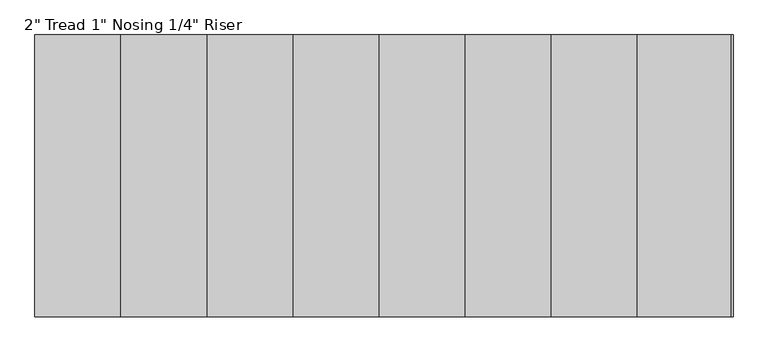
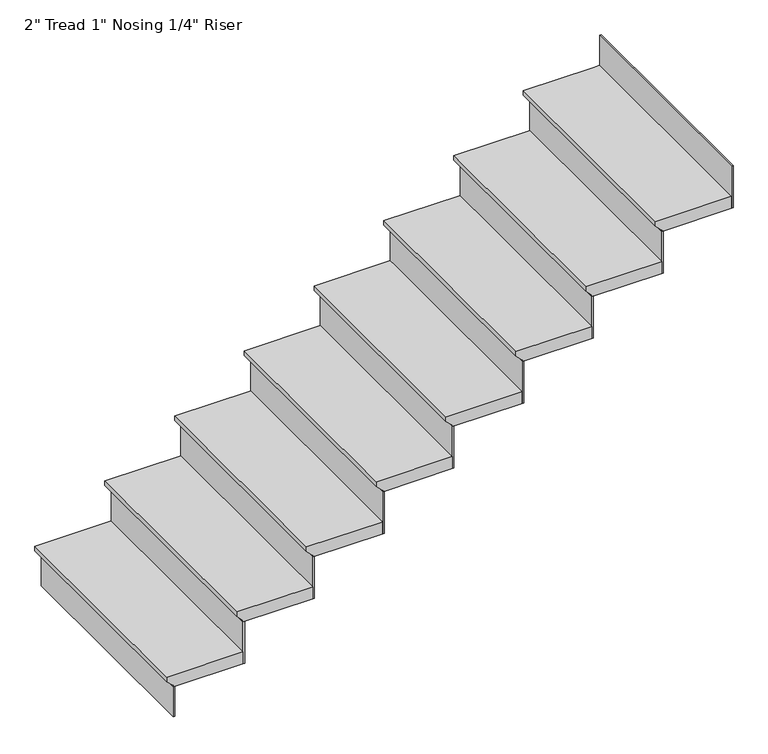
"""IFC4 building model written with IfcOpenShell, lengths in millimetres: stair flight geometry."""

from ifc_helpers import new_model, si_unit, origin, place, context, project, spatial, faceted_brep, source, transform, mapped, element, save


def stair_flight_350f2e97(model_context):
    return source(origin(), model_context, "Body", "Brep", [
        faceted_brep([(-4413.813859, 444.1428136, 158.75), (-4413.813859, 444.1428136, 177.8), (-4413.813859, 1358.5428136, 177.8), (-4413.813859, 1358.5428136, 158.75), (-4388.413859, 444.1428136, 133.35), (-4388.413859, 1358.5428136, 133.35), (-4109.013859, 444.1428136, 177.8), (-4109.013859, 1358.5428136, 177.8), (-4388.413859, 1358.5428136, 127.0), (-4109.013859, 1358.5428136, 127.0), (-4109.013859, 444.1428136, 127.0), (-4388.413859, 444.1428136, 127.0)], [[[0, 1, 2, 3]], [[4, 0, 3, 5]], [[2, 1, 6, 7]], [[8, 9, 10, 11]], [[2, 7, 9, 8, 5, 3]], [[8, 11, 4, 5]], [[6, 1, 0, 4, 11, 10]], [[7, 6, 10, 9]]]),
        faceted_brep([(-4388.413859, 444.1428136, 127.0), (-4388.413859, 444.1428136, 0.0), (-4382.063859, 444.1428136, 0.0), (-4382.063859, 444.1428136, 127.0), (-4388.413859, 1358.5428136, 127.0), (-4382.063859, 1358.5428136, 127.0), (-4382.063859, 1358.5428136, 0.0), (-4388.413859, 1358.5428136, 0.0)], [[[0, 1, 2, 3]], [[4, 5, 6, 7]], [[1, 0, 4, 7]], [[2, 1, 7, 6]], [[3, 2, 6, 5]], [[0, 3, 5, 4]]]),
        faceted_brep([(-4109.013859, 444.1428136, 304.8), (-4109.013859, 444.1428136, 127.0), (-4102.663859, 444.1428136, 127.0), (-4102.663859, 444.1428136, 304.8), (-4109.013859, 1358.5428136, 304.8), (-4102.663859, 1358.5428136, 304.8), (-4102.663859, 1358.5428136, 127.0), (-4109.013859, 1358.5428136, 127.0)], [[[0, 1, 2, 3]], [[4, 5, 6, 7]], [[1, 0, 4, 7]], [[2, 1, 7, 6]], [[3, 2, 6, 5]], [[0, 3, 5, 4]]]),
        faceted_brep([(-4134.413859, 1358.5428136, 355.6), (-4134.413859, 444.1428136, 355.6), (-3829.613859, 444.1428136, 355.6), (-3829.613859, 1358.5428136, 355.6), (-4109.013859, 1358.5428136, 304.8), (-3829.613859, 1358.5428136, 304.8), (-3829.613859, 444.1428136, 304.8), (-4109.013859, 444.1428136, 304.8), (-4109.013859, 1358.5428136, 311.15), (-4134.413859, 1358.5428136, 336.55), (-4109.013859, 444.1428136, 311.15), (-4134.413859, 444.1428136, 336.55)], [[[0, 1, 2, 3]], [[4, 5, 6, 7]], [[0, 3, 5, 4, 8, 9]], [[4, 7, 10, 8]], [[2, 1, 11, 10, 7, 6]], [[3, 2, 6, 5]], [[11, 1, 0, 9]], [[10, 11, 9, 8]]]),
        faceted_brep([(-3829.613859, 444.1428136, 482.6), (-3829.613859, 444.1428136, 304.8), (-3823.263859, 444.1428136, 304.8), (-3823.263859, 444.1428136, 482.6), (-3829.613859, 1358.5428136, 482.6), (-3823.263859, 1358.5428136, 482.6), (-3823.263859, 1358.5428136, 304.8), (-3829.613859, 1358.5428136, 304.8)], [[[0, 1, 2, 3]], [[4, 5, 6, 7]], [[1, 0, 4, 7]], [[2, 1, 7, 6]], [[3, 2, 6, 5]], [[0, 3, 5, 4]]]),
        faceted_brep([(-3855.013859, 1358.5428136, 533.4), (-3855.013859, 444.1428136, 533.4), (-3550.213859, 444.1428136, 533.4), (-3550.213859, 1358.5428136, 533.4), (-3829.613859, 1358.5428136, 482.6), (-3550.213859, 1358.5428136, 482.6), (-3550.213859, 444.1428136, 482.6), (-3829.613859, 444.1428136, 482.6), (-3829.613859, 1358.5428136, 488.95), (-3855.013859, 1358.5428136, 514.35), (-3829.613859, 444.1428136, 488.95), (-3855.013859, 444.1428136, 514.35)], [[[0, 1, 2, 3]], [[4, 5, 6, 7]], [[0, 3, 5, 4, 8, 9]], [[4, 7, 10, 8]], [[2, 1, 11, 10, 7, 6]], [[3, 2, 6, 5]], [[11, 1, 0, 9]], [[10, 11, 9, 8]]]),
        faceted_brep([(-3550.213859, 444.1428136, 660.4), (-3550.213859, 444.1428136, 482.6), (-3543.863859, 444.1428136, 482.6), (-3543.863859, 444.1428136, 660.4), (-3550.213859, 1358.5428136, 660.4), (-3543.863859, 1358.5428136, 660.4), (-3543.863859, 1358.5428136, 482.6), (-3550.213859, 1358.5428136, 482.6)], [[[0, 1, 2, 3]], [[4, 5, 6, 7]], [[1, 0, 4, 7]], [[2, 1, 7, 6]], [[3, 2, 6, 5]], [[0, 3, 5, 4]]]),
        faceted_brep([(-3575.613859, 1358.5428136, 711.2), (-3575.613859, 444.1428136, 711.2), (-3270.813859, 444.1428136, 711.2), (-3270.813859, 1358.5428136, 711.2), (-3550.213859, 1358.5428136, 660.4), (-3270.813859, 1358.5428136, 660.4), (-3270.813859, 444.1428136, 660.4), (-3550.213859, 444.1428136, 660.4), (-3550.213859, 1358.5428136, 666.75), (-3575.613859, 1358.5428136, 692.15), (-3550.213859, 444.1428136, 666.75), (-3575.613859, 444.1428136, 692.15)], [[[0, 1, 2, 3]], [[4, 5, 6, 7]], [[0, 3, 5, 4, 8, 9]], [[4, 7, 10, 8]], [[2, 1, 11, 10, 7, 6]], [[3, 2, 6, 5]], [[11, 1, 0, 9]], [[10, 11, 9, 8]]]),
        faceted_brep([(-3270.813859, 444.1428136, 838.2), (-3270.813859, 444.1428136, 660.4), (-3264.463859, 444.1428136, 660.4), (-3264.463859, 444.1428136, 838.2), (-3270.813859, 1358.5428136, 838.2), (-3264.463859, 1358.5428136, 838.2), (-3264.463859, 1358.5428136, 660.4), (-3270.813859, 1358.5428136, 660.4)], [[[0, 1, 2, 3]], [[4, 5, 6, 7]], [[1, 0, 4, 7]], [[2, 1, 7, 6]], [[3, 2, 6, 5]], [[0, 3, 5, 4]]]),
        faceted_brep([(-3296.213859, 1358.5428136, 889.0), (-3296.213859, 444.1428136, 889.0), (-2991.413859, 444.1428136, 889.0), (-2991.413859, 1358.5428136, 889.0), (-3270.813859, 1358.5428136, 838.2), (-2991.413859, 1358.5428136, 838.2), (-2991.413859, 444.1428136, 838.2), (-3270.813859, 444.1428136, 838.2), (-3270.813859, 1358.5428136, 844.55), (-3296.213859, 1358.5428136, 869.95), (-3270.813859, 444.1428136, 844.55), (-3296.213859, 444.1428136, 869.95)], [[[0, 1, 2, 3]], [[4, 5, 6, 7]], [[0, 3, 5, 4, 8, 9]], [[4, 7, 10, 8]], [[2, 1, 11, 10, 7, 6]], [[3, 2, 6, 5]], [[11, 1, 0, 9]], [[10, 11, 9, 8]]]),
        faceted_brep([(-2991.413859, 444.1428136, 1016.0), (-2991.413859, 444.1428136, 838.2), (-2985.063859, 444.1428136, 838.2), (-2985.063859, 444.1428136, 1016.0), (-2991.413859, 1358.5428136, 1016.0), (-2985.063859, 1358.5428136, 1016.0), (-2985.063859, 1358.5428136, 838.2), (-2991.413859, 1358.5428136, 838.2)], [[[0, 1, 2, 3]], [[4, 5, 6, 7]], [[1, 0, 4, 7]], [[2, 1, 7, 6]], [[3, 2, 6, 5]], [[0, 3, 5, 4]]]),
        faceted_brep([(-3016.813859, 1358.5428136, 1066.8), (-3016.813859, 444.1428136, 1066.8), (-2712.013859, 444.1428136, 1066.8), (-2712.013859, 1358.5428136, 1066.8), (-2991.413859, 1358.5428136, 1016.0), (-2712.013859, 1358.5428136, 1016.0), (-2712.013859, 444.1428136, 1016.0), (-2991.413859, 444.1428136, 1016.0), (-2991.413859, 1358.5428136, 1022.35), (-3016.813859, 1358.5428136, 1047.75), (-2991.413859, 444.1428136, 1022.35), (-3016.813859, 444.1428136, 1047.75)], [[[0, 1, 2, 3]], [[4, 5, 6, 7]], [[0, 3, 5, 4, 8, 9]], [[4, 7, 10, 8]], [[2, 1, 11, 10, 7, 6]], [[3, 2, 6, 5]], [[11, 1, 0, 9]], [[10, 11, 9, 8]]]),
        faceted_brep([(-2712.013859, 444.1428136, 1193.8), (-2712.013859, 444.1428136, 1016.0), (-2705.663859, 444.1428136, 1016.0), (-2705.663859, 444.1428136, 1193.8), (-2712.013859, 1358.5428136, 1193.8), (-2705.663859, 1358.5428136, 1193.8), (-2705.663859, 1358.5428136, 1016.0), (-2712.013859, 1358.5428136, 1016.0)], [[[0, 1, 2, 3]], [[4, 5, 6, 7]], [[1, 0, 4, 7]], [[2, 1, 7, 6]], [[3, 2, 6, 5]], [[0, 3, 5, 4]]]),
        faceted_brep([(-2737.413859, 1358.5428136, 1244.6), (-2737.413859, 444.1428136, 1244.6), (-2432.613859, 444.1428136, 1244.6), (-2432.613859, 1358.5428136, 1244.6), (-2712.013859, 1358.5428136, 1193.8), (-2432.613859, 1358.5428136, 1193.8), (-2432.613859, 444.1428136, 1193.8), (-2712.013859, 444.1428136, 1193.8), (-2712.013859, 1358.5428136, 1200.15), (-2737.413859, 1358.5428136, 1225.55), (-2712.013859, 444.1428136, 1200.15), (-2737.413859, 444.1428136, 1225.55)], [[[0, 1, 2, 3]], [[4, 5, 6, 7]], [[0, 3, 5, 4, 8, 9]], [[4, 7, 10, 8]], [[2, 1, 11, 10, 7, 6]], [[3, 2, 6, 5]], [[11, 1, 0, 9]], [[10, 11, 9, 8]]]),
        faceted_brep([(-2153.213859, 444.1428136, 1549.4), (-2153.213859, 444.1428136, 1371.6), (-2146.863859, 444.1428136, 1371.6), (-2146.863859, 444.1428136, 1549.4), (-2153.213859, 1358.5428136, 1549.4), (-2146.863859, 1358.5428136, 1549.4), (-2146.863859, 1358.5428136, 1371.6), (-2153.213859, 1358.5428136, 1371.6)], [[[0, 1, 2, 3]], [[4, 5, 6, 7]], [[1, 0, 4, 7]], [[2, 1, 7, 6]], [[3, 2, 6, 5]], [[0, 3, 5, 4]]]),
        faceted_brep([(-2432.613859, 444.1428136, 1371.6), (-2432.613859, 444.1428136, 1193.8), (-2426.263859, 444.1428136, 1193.8), (-2426.263859, 444.1428136, 1371.6), (-2432.613859, 1358.5428136, 1371.6), (-2426.263859, 1358.5428136, 1371.6), (-2426.263859, 1358.5428136, 1193.8), (-2432.613859, 1358.5428136, 1193.8)], [[[0, 1, 2, 3]], [[4, 5, 6, 7]], [[1, 0, 4, 7]], [[2, 1, 7, 6]], [[3, 2, 6, 5]], [[0, 3, 5, 4]]]),
        faceted_brep([(-2153.213859, 1358.5428136, 1422.4), (-2178.613859, 1358.5428136, 1422.4), (-2458.013859, 1358.5428136, 1422.4), (-2458.013859, 444.1428136, 1422.4), (-2153.213859, 444.1428136, 1422.4), (-2178.613859, 1358.5428136, 1371.6), (-2153.213859, 1358.5428136, 1371.6), (-2153.213859, 444.1428136, 1371.6), (-2432.613859, 444.1428136, 1371.6), (-2432.613859, 1358.5428136, 1371.6), (-2432.613859, 1358.5428136, 1377.95), (-2458.013859, 1358.5428136, 1403.35), (-2432.613859, 444.1428136, 1377.95), (-2458.013859, 444.1428136, 1403.35)], [[[0, 1, 2, 3, 4]], [[5, 6, 7, 8, 9]], [[1, 0, 6, 5]], [[2, 1, 5, 9, 10, 11]], [[9, 8, 12, 10]], [[4, 3, 13, 12, 8, 7]], [[0, 4, 7, 6]], [[13, 3, 2, 11]], [[12, 13, 11, 10]]]),
    ])


if __name__ == "__main__":
    model = new_model("IFC4")
    model_context = context("Model", 3, world=origin())
    ifc_project = project(units=[si_unit("LENGTHUNIT", "METRE", prefix="MILLI")], contexts=[model_context])
    site = spatial("IfcSite", under=ifc_project)
    building = spatial("IfcBuilding", under=site)
    placement = place(None, origin())
    stair_flight_shape = stair_flight_350f2e97(model_context)
    element("IfcStairFlight", 1, ObjectType="2\" Tread 1\" Nosing 1/4\" Riser", at=placement, inside=building, context=model_context, shape_type="MappedRepresentation", body=[
        mapped(stair_flight_shape, transform((0.0, 0.0, 0.0), x_axis=(1.0, 0.0, 0.0), y_axis=(0.0, 1.0, 0.0), z_axis=(0.0, 0.0, 1.0))),
    ])
    save(model, "model.ifc")
